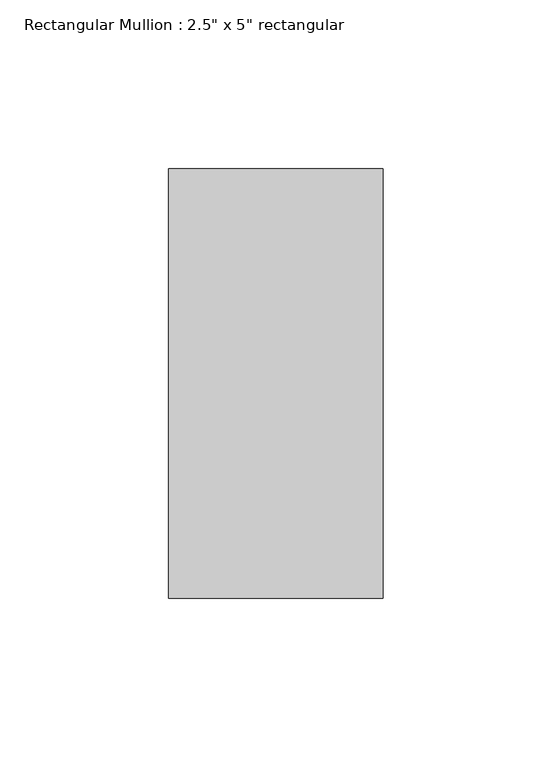
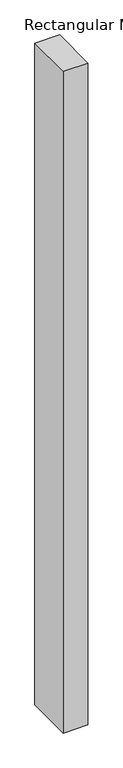
"""IFC4 building model written with IfcOpenShell, lengths in millimetres: member geometry."""

from ifc_helpers import new_model, si_unit, frame, origin, place, context, project, spatial, polyline, outline, extrude, source, transform, mapped, element, save


def member_337b6441(model_context):
    return source(origin(), model_context, "Body", "SweptSolid", [
        extrude(outline(polyline([(31.75, 63.5), (31.75, -63.5), (-31.75, -63.5), (-31.75, 63.5), (31.75, 63.5)])), frame((0.0, 0.0, -1805.4265918), z_axis=(0.0, 0.0, 1.0), x_axis=(1.0, 0.0, 0.0)), (0.0, 0.0, 1.0), 1805.4265918),
    ])


if __name__ == "__main__":
    model = new_model("IFC4")
    model_context = context("Model", 3, world=origin())
    ifc_project = project(units=[si_unit("LENGTHUNIT", "METRE", prefix="MILLI")], contexts=[model_context])
    site = spatial("IfcSite", under=ifc_project)
    building = spatial("IfcBuilding", under=site)
    placement = place(None, origin())
    member_shape = member_337b6441(model_context)
    element("IfcMember", 1, ObjectType="Rectangular Mullion : 2.5\" x 5\" rectangular", at=placement, inside=building, context=model_context, shape_type="MappedRepresentation", body=[
        mapped(member_shape, transform((0.0, 0.0, 0.0), x_axis=(1.0, 0.0, 0.0), y_axis=(0.0, 1.0, 0.0), z_axis=(0.0, 0.0, 1.0))),
    ])
    save(model, "model.ifc")

# Revit data of these elements
# Type "Rectangular Mullion : 2.5\" x 5\" rectangular"
#   built-in parameter 1007304 = 0.416667 (stored number, unit not read)
#   built-in parameter 1007301 = 0.104167 (stored number, unit not read)
#   built-in parameter 1007300 = 0.104167 (stored number, unit not read)
# Element 1 (IfcMember, "Rectangular Mullion : 2.5\" x 5\" rectangular")
#   Materials on its faces: "Aluminum"
# Materials
#   "Aluminum": class "Metal", colour RGB 247 247 247, transparency 0, Description = "Aluminum 6061", Cost = 0
